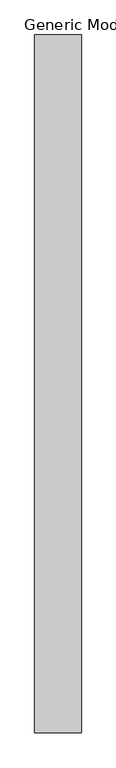
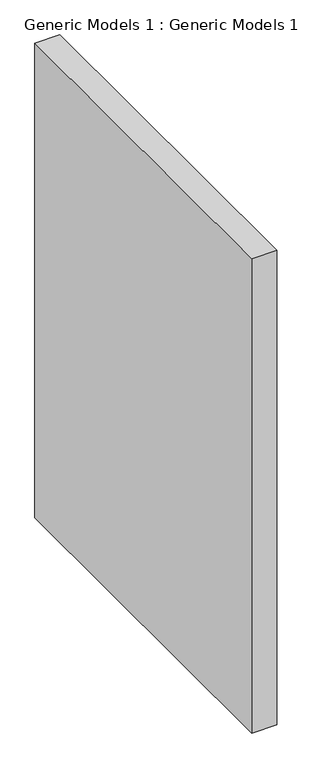
"""IFC4 building model written with IfcOpenShell, lengths in millimetres: proxy geometry, Generic Models 1 : Generic Models 1."""

from ifc_helpers import new_model, si_unit, frame, origin, place, context, project, spatial, polyline, outline, extrude, source, transform, mapped, element, save


def generic_models_1_generic_models_1_b00c282c(model_context):
    return source(origin(), model_context, "Body", "SweptSolid", [
        extrude(outline(polyline([(2881.8546869, -4272.2938352), (2881.8546869, -6552.5533764), (2729.4546869, -6552.5533764), (2729.4546869, -4272.2938352), (2881.8546869, -4272.2938352)])), frame((0.0, 0.0, 3352.8), z_axis=(0.0, 0.0, 1.0), x_axis=(1.0, 0.0, 0.0)), (0.0, 0.0, 1.0), 3048.0),
    ])


if __name__ == "__main__":
    model = new_model("IFC4")
    model_context = context("Model", 3, world=origin())
    ifc_project = project(units=[si_unit("LENGTHUNIT", "METRE", prefix="MILLI")], contexts=[model_context])
    site = spatial("IfcSite", under=ifc_project)
    building = spatial("IfcBuilding", under=site)
    placement = place(None, origin())
    generic_models_1_generic_models_1_shape = generic_models_1_generic_models_1_b00c282c(model_context)
    element("IfcBuildingElementProxy", 1, Name="Generic Models 1 : Generic Models 1", ObjectType="Generic Models 1 : Generic Models 1", at=placement, inside=building, context=model_context, shape_type="MappedRepresentation", body=[
        mapped(generic_models_1_generic_models_1_shape, transform((0.0, 0.0, 0.0), x_axis=(1.0, 0.0, 0.0), y_axis=(0.0, 1.0, 0.0), z_axis=(0.0, 0.0, 1.0))),
    ])
    save(model, "model.ifc")

# Revit data of these elements
# Element 1 (IfcBuildingElementProxy, "Generic Models 1 : Generic Models 1")
#   Materials on its faces: "WALL PAINT"
# Materials
#   "WALL PAINT": class "Generic", colour RGB 120 120 120, transparency 0, Cost = 0
